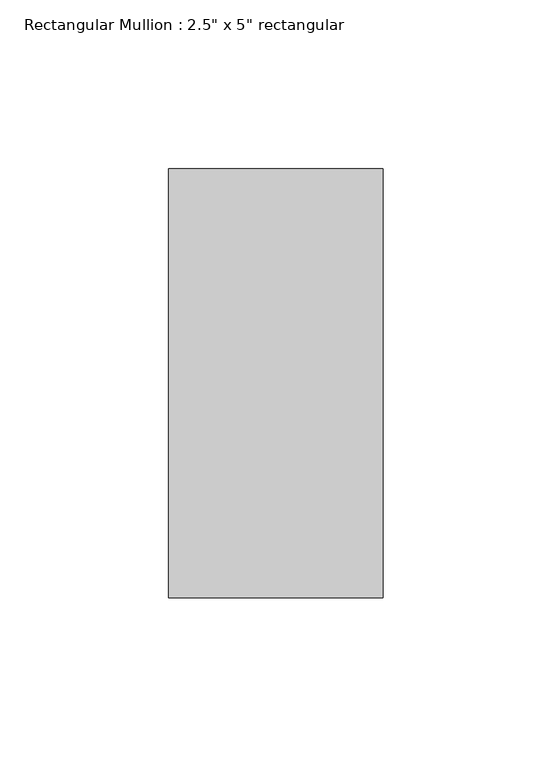
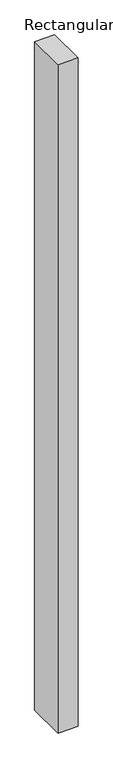
"""IFC4 building model written with IfcOpenShell, lengths in millimetres: member geometry."""

from ifc_helpers import new_model, si_unit, frame, origin, place, context, project, spatial, polyline, outline, extrude, source, transform, mapped, element, save


def member_d1708325(model_context):
    return source(origin(), model_context, "Body", "SweptSolid", [
        extrude(outline(polyline([(0.0, 63.5), (0.0, -63.5), (-63.5, -63.5), (-63.5, 63.5), (0.0, 63.5)])), frame((0.0, 0.0, -2235.2), z_axis=(0.0, 0.0, 1.0), x_axis=(1.0, 0.0, 0.0)), (0.0, 0.0, 1.0), 2235.2),
    ])


if __name__ == "__main__":
    model = new_model("IFC4")
    model_context = context("Model", 3, world=origin())
    ifc_project = project(units=[si_unit("LENGTHUNIT", "METRE", prefix="MILLI")], contexts=[model_context])
    site = spatial("IfcSite", under=ifc_project)
    building = spatial("IfcBuilding", under=site)
    placement = place(None, origin())
    member_shape = member_d1708325(model_context)
    element("IfcMember", 1, ObjectType="Rectangular Mullion : 2.5\" x 5\" rectangular", at=placement, inside=building, context=model_context, shape_type="MappedRepresentation", body=[
        mapped(member_shape, transform((0.0, 0.0, 0.0), x_axis=(1.0, 0.0, 0.0), y_axis=(0.0, 1.0, 0.0), z_axis=(0.0, 0.0, 1.0))),
    ])
    save(model, "model.ifc")

# Revit data of these elements
# Type "Rectangular Mullion : 2.5\" x 5\" rectangular"
#   built-in parameter 1007304 = 0.416667 (stored number, unit not read)
#   built-in parameter 1007301 = 0.104167 (stored number, unit not read)
#   built-in parameter 1007300 = 0.104167 (stored number, unit not read)
# Element 1 (IfcMember, "Rectangular Mullion : 2.5\" x 5\" rectangular")
#   Materials on its faces: "Aluminum"
# Materials
#   "Aluminum": class "Metal", colour RGB 247 247 247, transparency 0, Description = "Aluminum 6061", Cost = 0
